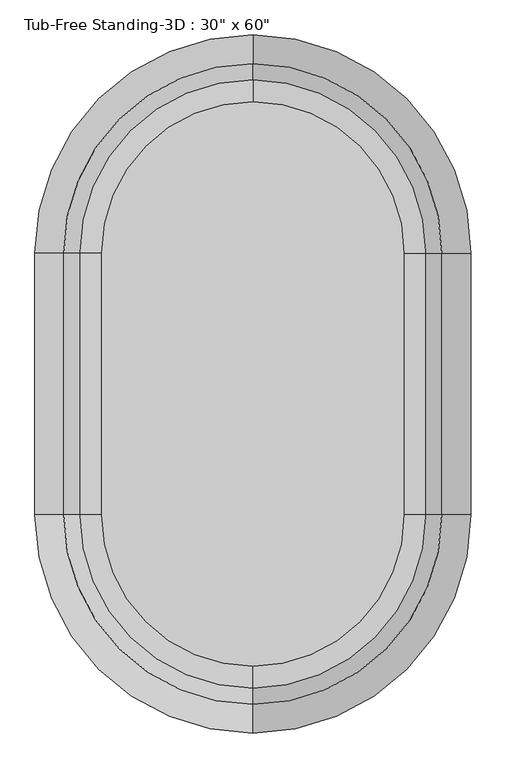
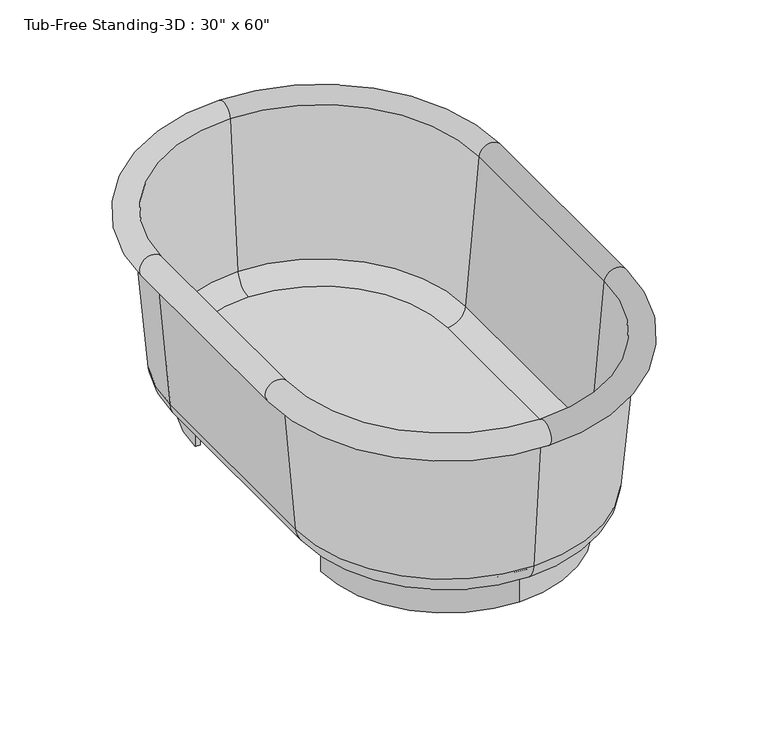
"""IFC4 building model written with IfcOpenShell, lengths in millimetres: flow terminal geometry."""

from ifc_helpers import new_model, si_unit, point, frame, frame_2d, origin, origin_with_axes, place, context, project, spatial, polyline, circle_curve, ellipse_curve, trimmed, segment, composite_curve, outline, extrude, source, transform, mapped, element, save
from ifc_brep_helpers import plane_surface, cylinder_surface, revolved_surface, advanced_brep


def flow_terminal_04541809(model_context):
    return source(origin(), model_context, "Body", "SolidModel", [
        extrude(outline(composite_curve([segment(trimmed(circle_curve(frame_2d((0.0, 228.6)), 254.0), [point((0.0, 482.6))], [point((-254.0, 228.6))], True, "CARTESIAN"), True, "CONTINUOUS"), segment(polyline([(-254.0, 228.6), (-264.2824236, 228.6)]), True, "CONTINUOUS"), segment(trimmed(circle_curve(frame_2d((0.0, 228.6)), 264.2824236), [point((-264.2824236, 228.6))], [point((0.0, 492.8824236))], False, "CARTESIAN"), True, "CONTINUOUS"), segment(trimmed(circle_curve(frame_2d((0.0, 228.6)), 264.2824236), [point((0.0, 492.8824236))], [point((264.2824236, 228.6))], False, "CARTESIAN"), True, "CONTINUOUS"), segment(polyline([(264.2824236, 228.6), (254.0, 228.6)]), True, "CONTINUOUS"), segment(trimmed(circle_curve(frame_2d((0.0, 228.6)), 254.0), [point((254.0, 228.6))], [point((0.0, 482.6))], True, "CARTESIAN"), True, "CONTINUOUS")], self_intersect=False)), origin_with_axes(), (0.0, 0.0, 1.0), 63.5),
        extrude(outline(composite_curve([segment(trimmed(circle_curve(frame_2d((0.0, -228.6)), 264.2824236), [point((0.0, -492.8824236))], [point((-264.2824236, -228.6))], False, "CARTESIAN"), True, "CONTINUOUS"), segment(polyline([(-264.2824236, -228.6), (-254.0, -228.6)]), True, "CONTINUOUS"), segment(trimmed(circle_curve(frame_2d((0.0, -228.6)), 254.0), [point((-254.0, -228.6))], [point((0.0, -482.6))], True, "CARTESIAN"), True, "CONTINUOUS"), segment(trimmed(circle_curve(frame_2d((0.0, -228.6)), 254.0), [point((0.0, -482.6))], [point((254.0, -228.6))], True, "CARTESIAN"), True, "CONTINUOUS"), segment(polyline([(254.0, -228.6), (264.2824236, -228.6)]), True, "CONTINUOUS"), segment(trimmed(circle_curve(frame_2d((0.0, -228.6)), 264.2824236), [point((264.2824236, -228.6))], [point((0.0, -492.8824236))], False, "CARTESIAN"), True, "CONTINUOUS")], self_intersect=False)), origin_with_axes(), (0.0, 0.0, 1.0), 63.5),
        extrude(outline(composite_curve([segment(polyline([(-264.2824236, -228.6), (-264.2824236, 228.6)]), True, "CONTINUOUS"), segment(trimmed(circle_curve(frame_2d((0.0, 228.6)), 264.2824236), [point((-264.2824236, 228.6))], [point((0.0, 492.8824236))], False, "CARTESIAN"), True, "CONTINUOUS"), segment(trimmed(circle_curve(frame_2d((0.0, 228.6)), 264.2824236), [point((0.0, 492.8824236))], [point((264.2824236, 228.6))], False, "CARTESIAN"), True, "CONTINUOUS"), segment(polyline([(264.2824236, 228.6), (264.2824236, -228.6)]), True, "CONTINUOUS"), segment(trimmed(circle_curve(frame_2d((0.0, -228.6)), 264.2824236), [point((264.2824236, -228.6))], [point((0.0, -492.8824236))], False, "CARTESIAN"), True, "CONTINUOUS"), segment(trimmed(circle_curve(frame_2d((0.0, -228.6)), 264.2824236), [point((0.0, -492.8824236))], [point((-264.2824236, -228.6))], False, "CARTESIAN"), True, "CONTINUOUS")], self_intersect=False)), frame((0.0, 0.0, 63.5), z_axis=(0.0, 0.0, 1.0), x_axis=(1.0, 0.0, 0.0)), (0.0, 0.0, 1.0), 15.08125),
        advanced_brep(
        [(0.0, -571.5, 406.4), (342.9, -228.6, 406.4), (355.6, -228.6, 406.4), (0.0, -584.2, 406.4), (0.0, -545.7045038, 111.5561295), (317.1045038, -228.6, 111.5561295), (0.0, -492.8824236, 63.1536107), (264.2824236, -228.6, 63.1536107), (0.0, -492.8824236, 78.0774627), (264.2824236, -228.6, 78.0774627), (0.0, -530.8374416, 112.8568289), (302.2374416, -228.6, 112.8568289), (0.0, -559.0561556, 435.3982063), (330.4561556, -228.6, 435.3982063), (-342.9, -228.6, 406.4), (-355.6, -228.6, 406.4), (-317.1045038, -228.6, 111.5561295), (-264.2824236, -228.6, 63.1536107), (-264.2824236, -228.6, 78.0774627), (-302.2374416, -228.6, 112.8568289), (-330.4561556, -228.6, 435.3982063), (-355.6, 228.6, 406.4), (-342.9, 228.6, 406.4), (-317.1045038, 228.6, 111.5561295), (-264.2824236, 228.6, 63.1536107), (-264.2824236, 228.6, 78.0774627), (-302.2374416, 228.6, 112.8568289), (-330.4561556, 228.6, 435.3982063), (0.0, 571.5, 406.4), (0.0, 584.2, 406.4), (0.0, 545.7045038, 111.5561295), (0.0, 492.8824236, 63.1536107), (0.0, 492.8824236, 78.0774627), (0.0, 530.8374416, 112.8568289), (0.0, 559.0561556, 435.3982063), (342.9, 228.6, 406.4), (355.6, 228.6, 406.4), (317.1045038, 228.6, 111.5561295), (264.2824236, 228.6, 63.1536107), (264.2824236, 228.6, 78.0774627), (302.2374416, 228.6, 112.8568289), (330.4561556, 228.6, 435.3982063)],
        [
            (0, 1, circle_curve(frame((0.0, -228.6, 406.4), z_axis=(0.0, 0.0, 1.0), x_axis=(1.0, 0.0, 0.0)), 342.9)),
            (1, 2),
            (2, 3, circle_curve(frame((0.0, -228.6, 406.4), z_axis=(0.0, 0.0, -1.0), x_axis=(1.0, 0.0, 0.0)), 355.6)),
            (3, 0),
            (4, 5, circle_curve(frame((0.0, -228.6, 111.5561295), z_axis=(0.0, 0.0, 1.0), x_axis=(1.0, 0.0, 0.0)), 317.1045038)),
            (5, 1),
            (0, 4),
            (6, 7, circle_curve(frame((0.0, -228.6, 63.1536107), z_axis=(0.0, 0.0, 1.0), x_axis=(1.0, 0.0, 0.0)), 264.2824236)),
            (7, 5, circle_curve(frame((264.2824236, -228.6, 116.1774627), z_axis=(0.0, -1.0, 0.0), x_axis=(1.0, 0.0, 0.0)), 53.023852)),
            (4, 6, circle_curve(frame((0.0, -492.8824236, 116.1774627), z_axis=(1.0, 0.0, 0.0), x_axis=(0.0, -1.0, 0.0)), 53.023852)),
            (8, 9, circle_curve(frame((0.0, -228.6, 78.0774627), z_axis=(0.0, 0.0, 1.0), x_axis=(1.0, 0.0, 0.0)), 264.2824236)),
            (9, 7),
            (6, 8),
            (10, 11, circle_curve(frame((0.0, -228.6, 112.8568289), z_axis=(0.0, 0.0, 1.0), x_axis=(1.0, 0.0, 0.0)), 302.2374416)),
            (11, 9, circle_curve(frame((264.2824236, -228.6, 116.1774627), z_axis=(0.0, 1.0, 0.0), x_axis=(1.0, 0.0, 0.0)), 38.1)),
            (8, 10, circle_curve(frame((0.0, -492.8824236, 116.1774627), z_axis=(-1.0, 0.0, 0.0), x_axis=(0.0, -1.0, 0.0)), 38.1)),
            (12, 13, circle_curve(frame((0.0, -228.6, 435.3982063), z_axis=(0.0, 0.0, 1.0), x_axis=(1.0, 0.0, 0.0)), 330.4561556)),
            (13, 11),
            (10, 12),
            (2, 13, circle_curve(frame((355.6, -228.6, 431.8), z_axis=(0.0, -1.0, 0.0), x_axis=(1.0, 0.0, 0.0)), 25.4)),
            (12, 3, circle_curve(frame((0.0, -584.2, 431.8), z_axis=(1.0, 0.0, 0.0), x_axis=(0.0, -1.0, 0.0)), 25.4)),
            (14, 0, circle_curve(frame((0.0, -228.6, 406.4), z_axis=(0.0, 0.0, 1.0), x_axis=(0.0, -1.0, 0.0)), 342.9)),
            (3, 15, circle_curve(frame((0.0, -228.6, 406.4), z_axis=(0.0, 0.0, -1.0), x_axis=(0.0, -1.0, 0.0)), 355.6)),
            (15, 14),
            (16, 4, circle_curve(frame((0.0, -228.6, 111.5561295), z_axis=(0.0, 0.0, 1.0), x_axis=(0.0, -1.0, 0.0)), 317.1045038)),
            (14, 16),
            (17, 6, circle_curve(frame((0.0, -228.6, 63.1536107), z_axis=(0.0, 0.0, 1.0), x_axis=(0.0, -1.0, 0.0)), 264.2824236)),
            (16, 17, circle_curve(frame((-264.2824236, -228.6, 116.1774627), z_axis=(0.0, -1.0, 0.0), x_axis=(-1.0, 0.0, 0.0)), 53.023852)),
            (18, 8, circle_curve(frame((0.0, -228.6, 78.0774627), z_axis=(0.0, 0.0, 1.0), x_axis=(0.0, -1.0, 0.0)), 264.2824236)),
            (17, 18),
            (19, 10, circle_curve(frame((0.0, -228.6, 112.8568289), z_axis=(0.0, 0.0, 1.0), x_axis=(0.0, -1.0, 0.0)), 302.2374416)),
            (18, 19, circle_curve(frame((-264.2824236, -228.6, 116.1774627), z_axis=(0.0, 1.0, 0.0), x_axis=(-1.0, 0.0, 0.0)), 38.1)),
            (20, 12, circle_curve(frame((0.0, -228.6, 435.3982063), z_axis=(0.0, 0.0, 1.0), x_axis=(0.0, -1.0, 0.0)), 330.4561556)),
            (19, 20),
            (20, 15, circle_curve(frame((-355.6, -228.6, 431.8), z_axis=(0.0, -1.0, 0.0), x_axis=(-1.0, 0.0, 0.0)), 25.4)),
            (15, 21),
            (21, 22),
            (22, 14),
            (22, 23),
            (23, 16),
            (23, 24, circle_curve(frame((-264.2824236, 228.6, 116.1774627), z_axis=(0.0, -1.0, 0.0), x_axis=(-1.0, 0.0, 0.0)), 53.023852)),
            (24, 17),
            (24, 25),
            (25, 18),
            (25, 26, circle_curve(frame((-264.2824236, 228.6, 116.1774627), z_axis=(0.0, 1.0, 0.0), x_axis=(-1.0, 0.0, 0.0)), 38.1)),
            (26, 19),
            (26, 27),
            (27, 20),
            (27, 21, circle_curve(frame((-355.6, 228.6, 431.8), z_axis=(0.0, -1.0, 0.0), x_axis=(-1.0, 0.0, 0.0)), 25.4)),
            (28, 22, circle_curve(frame((0.0, 228.6, 406.4), z_axis=(0.0, 0.0, 1.0), x_axis=(-1.0, 0.0, 0.0)), 342.9)),
            (21, 29, circle_curve(frame((0.0, 228.6, 406.4), z_axis=(0.0, 0.0, -1.0), x_axis=(-1.0, 0.0, 0.0)), 355.6)),
            (29, 28),
            (30, 23, circle_curve(frame((0.0, 228.6, 111.5561295), z_axis=(0.0, 0.0, 1.0), x_axis=(-1.0, 0.0, 0.0)), 317.1045038)),
            (28, 30),
            (31, 24, circle_curve(frame((0.0, 228.6, 63.1536107), z_axis=(0.0, 0.0, 1.0), x_axis=(-1.0, 0.0, 0.0)), 264.2824236)),
            (30, 31, circle_curve(frame((0.0, 492.8824236, 116.1774627), z_axis=(-1.0, 0.0, 0.0), x_axis=(0.0, 1.0, 0.0)), 53.023852)),
            (32, 25, circle_curve(frame((0.0, 228.6, 78.0774627), z_axis=(0.0, 0.0, 1.0), x_axis=(-1.0, 0.0, 0.0)), 264.2824236)),
            (31, 32),
            (33, 26, circle_curve(frame((0.0, 228.6, 112.8568289), z_axis=(0.0, 0.0, 1.0), x_axis=(-1.0, 0.0, 0.0)), 302.2374416)),
            (32, 33, circle_curve(frame((0.0, 492.8824236, 116.1774627), z_axis=(1.0, 0.0, 0.0), x_axis=(0.0, 1.0, 0.0)), 38.1)),
            (34, 27, circle_curve(frame((0.0, 228.6, 435.3982063), z_axis=(0.0, 0.0, 1.0), x_axis=(-1.0, 0.0, 0.0)), 330.4561556)),
            (33, 34),
            (34, 29, circle_curve(frame((0.0, 584.2, 431.8), z_axis=(-1.0, 0.0, 0.0), x_axis=(0.0, 1.0, 0.0)), 25.4)),
            (35, 28, circle_curve(frame((0.0, 228.6, 406.4), z_axis=(0.0, 0.0, 1.0), x_axis=(0.0, 1.0, 0.0)), 342.9)),
            (29, 36, circle_curve(frame((0.0, 228.6, 406.4), z_axis=(0.0, 0.0, -1.0), x_axis=(0.0, 1.0, 0.0)), 355.6)),
            (36, 35),
            (37, 30, circle_curve(frame((0.0, 228.6, 111.5561295), z_axis=(0.0, 0.0, 1.0), x_axis=(0.0, 1.0, 0.0)), 317.1045038)),
            (35, 37),
            (38, 31, circle_curve(frame((0.0, 228.6, 63.1536107), z_axis=(0.0, 0.0, 1.0), x_axis=(0.0, 1.0, 0.0)), 264.2824236)),
            (37, 38, circle_curve(frame((264.2824236, 228.6, 116.1774627), z_axis=(0.0, 1.0, 0.0), x_axis=(1.0, 0.0, 0.0)), 53.023852)),
            (39, 32, circle_curve(frame((0.0, 228.6, 78.0774627), z_axis=(0.0, 0.0, 1.0), x_axis=(0.0, 1.0, 0.0)), 264.2824236)),
            (38, 39),
            (40, 33, circle_curve(frame((0.0, 228.6, 112.8568289), z_axis=(0.0, 0.0, 1.0), x_axis=(0.0, 1.0, 0.0)), 302.2374416)),
            (39, 40, circle_curve(frame((264.2824236, 228.6, 116.1774627), z_axis=(0.0, -1.0, 0.0), x_axis=(1.0, 0.0, 0.0)), 38.1)),
            (41, 34, circle_curve(frame((0.0, 228.6, 435.3982063), z_axis=(0.0, 0.0, 1.0), x_axis=(0.0, 1.0, 0.0)), 330.4561556)),
            (40, 41),
            (41, 36, circle_curve(frame((355.6, 228.6, 431.8), z_axis=(0.0, 1.0, 0.0), x_axis=(1.0, 0.0, 0.0)), 25.4)),
            (36, 2),
            (1, 35),
            (5, 37),
            (7, 38),
            (9, 39),
            (11, 40),
            (13, 41),
        ],
        [
            plane_surface(frame((0.0, -228.6, 406.4), z_axis=(0.0, 0.0, -1.0), x_axis=(1.0, 0.0, 0.0))),
            revolved_surface(polyline([(342.9, -228.6, 406.4), (317.1045038, -228.6, 111.5561295)]), (0.0, -228.6, 431.8), (0.0, 0.0, -1.0)),
            revolved_surface(trimmed(ellipse_curve(frame((264.2824236, -228.6, 116.1774627), z_axis=(0.0, 1.0, 0.0), x_axis=(1.0, 0.0, 0.0)), 53.023852, 53.023852), [point((317.1045038, -228.6, 111.5561295))], [point((264.2824236, -228.6, 63.1536107))], True, "CARTESIAN"), (0.0, -228.6, 431.8), (0.0, 0.0, -1.0)),
            revolved_surface(polyline([(264.2824236, -228.6, 63.1536107), (264.2824236, -228.6, 78.07746270000001)]), (0.0, -228.6, 431.8), (0.0, 0.0, -1.0)),
            revolved_surface(trimmed(ellipse_curve(frame((264.2824236, -228.6, 116.1774627), z_axis=(0.0, -1.0, 0.0), x_axis=(1.0, 0.0, 0.0)), 38.1, 38.1), [point((264.2824236, -228.6, 78.0774627))], [point((302.2374416, -228.6, 112.8568289))], True, "CARTESIAN"), (0.0, -228.6, 431.8), (0.0, 0.0, -1.0)),
            revolved_surface(polyline([(302.2374416, -228.6, 112.8568289), (330.4561556, -228.6, 435.3982063)]), (0.0, -228.6, 431.8), (0.0, 0.0, -1.0)),
            revolved_surface(trimmed(ellipse_curve(frame((355.6, -228.6, 431.8), z_axis=(0.0, 1.0, 0.0), x_axis=(1.0, 0.0, 0.0)), 25.4, 25.4), [point((330.4561556, -228.6, 435.3982063))], [point((355.6, -228.6, 406.4))], True, "CARTESIAN"), (0.0, -228.6, 431.8), (0.0, 0.0, -1.0)),
            plane_surface(frame((0.0, -228.6, 406.4), z_axis=(0.0, 0.0, -1.0), x_axis=(0.0, -1.0, 0.0))),
            revolved_surface(polyline([(0.0, -571.5, 406.4), (0.0, -545.7045038, 111.5561295)]), (0.0, -228.6, 431.8), (0.0, 0.0, -1.0)),
            revolved_surface(trimmed(ellipse_curve(frame((0.0, -492.8824236, 116.1774627), z_axis=(1.0, 0.0, 0.0), x_axis=(0.0, -1.0, 0.0)), 53.023852, 53.023852), [point((0.0, -545.7045038, 111.5561295))], [point((0.0, -492.8824236, 63.1536107))], True, "CARTESIAN"), (0.0, -228.6, 431.8), (0.0, 0.0, -1.0)),
            revolved_surface(polyline([(0.0, -492.88242360000004, 63.1536107), (0.0, -492.88242360000004, 78.07746270000001)]), (0.0, -228.6, 431.8), (0.0, 0.0, -1.0)),
            revolved_surface(trimmed(ellipse_curve(frame((0.0, -492.8824236, 116.1774627), z_axis=(-1.0, 0.0, 0.0), x_axis=(0.0, -1.0, 0.0)), 38.1, 38.1), [point((0.0, -492.8824236, 78.0774627))], [point((0.0, -530.8374416, 112.8568289))], True, "CARTESIAN"), (0.0, -228.6, 431.8), (0.0, 0.0, -1.0)),
            revolved_surface(polyline([(0.0, -530.8374416, 112.8568289), (0.0, -559.0561556, 435.3982063)]), (0.0, -228.6, 431.8), (0.0, 0.0, -1.0)),
            revolved_surface(trimmed(ellipse_curve(frame((0.0, -584.2, 431.8), z_axis=(1.0, 0.0, 0.0), x_axis=(0.0, -1.0, 0.0)), 25.4, 25.4), [point((0.0, -559.0561556, 435.3982063))], [point((0.0, -584.2, 406.4))], True, "CARTESIAN"), (0.0, -228.6, 431.8), (0.0, 0.0, -1.0)),
            plane_surface(frame((-355.6, -228.6, 406.4), z_axis=(0.0, 0.0, -1.0), x_axis=(0.0, 1.0, 0.0))),
            plane_surface(frame((-342.9, -228.6, 406.4), z_axis=(-0.9961946980917455, 0.0, -0.08715574274765871), x_axis=(0.0, 1.0, 0.0))),
            cylinder_surface(frame((-264.2824236, -228.6, 116.1774627), z_axis=(0.0, -1.0, 0.0), x_axis=(-1.0, 0.0, 0.0)), 53.023852),
            plane_surface(frame((-264.2824236, -228.6, 63.1536107), z_axis=(1.0, 0.0, 0.0), x_axis=(0.0, 1.0, 0.0))),
            revolved_surface(polyline([(-302.38242360000004, 228.6, 116.1774627), (-302.38242360000004, -228.6, 116.1774627)]), (-264.2824236, -228.6, 116.1774627), (0.0, 1.0, 0.0)),
            plane_surface(frame((-302.2374416, -228.6, 112.8568289), z_axis=(0.9961946980917458, 0.0, 0.08715574274765651), x_axis=(0.0, 1.0, 0.0))),
            cylinder_surface(frame((-355.6, -228.6, 431.8), z_axis=(0.0, -1.0, 0.0), x_axis=(-1.0, 0.0, 0.0)), 25.4),
            plane_surface(frame((0.0, 228.6, 406.4), z_axis=(0.0, 0.0, -1.0), x_axis=(-1.0, 0.0, 0.0))),
            revolved_surface(polyline([(-342.9, 228.6, 406.4), (-317.1045038, 228.6, 111.5561295)]), (0.0, 228.6, 431.8), (0.0, 0.0, -1.0)),
            revolved_surface(trimmed(ellipse_curve(frame((-264.2824236, 228.6, 116.1774627), z_axis=(0.0, -1.0, 0.0), x_axis=(-1.0, 0.0, 0.0)), 53.023852, 53.023852), [point((-317.1045038, 228.6, 111.5561295))], [point((-264.2824236, 228.6, 63.1536107))], True, "CARTESIAN"), (0.0, 228.6, 431.8), (0.0, 0.0, -1.0)),
            revolved_surface(polyline([(-264.2824236, 228.6, 63.1536107), (-264.2824236, 228.6, 78.07746270000001)]), (0.0, 228.6, 431.8), (0.0, 0.0, -1.0)),
            revolved_surface(trimmed(ellipse_curve(frame((-264.2824236, 228.6, 116.1774627), z_axis=(0.0, 1.0, 0.0), x_axis=(-1.0, 0.0, 0.0)), 38.1, 38.1), [point((-264.2824236, 228.6, 78.0774627))], [point((-302.2374416, 228.6, 112.8568289))], True, "CARTESIAN"), (0.0, 228.6, 431.8), (0.0, 0.0, -1.0)),
            revolved_surface(polyline([(-302.2374416, 228.6, 112.8568289), (-330.4561556, 228.6, 435.3982063)]), (0.0, 228.6, 431.8), (0.0, 0.0, -1.0)),
            revolved_surface(trimmed(ellipse_curve(frame((-355.6, 228.6, 431.8), z_axis=(0.0, -1.0, 0.0), x_axis=(-1.0, 0.0, 0.0)), 25.4, 25.4), [point((-330.4561556, 228.6, 435.3982063))], [point((-355.6, 228.6, 406.4))], True, "CARTESIAN"), (0.0, 228.6, 431.8), (0.0, 0.0, -1.0)),
            plane_surface(frame((0.0, 228.6, 406.4), z_axis=(0.0, 0.0, -1.0), x_axis=(0.0, 1.0, 0.0))),
            revolved_surface(polyline([(0.0, 571.5, 406.4), (0.0, 545.7045038, 111.5561295)]), (0.0, 228.6, 431.8), (0.0, 0.0, -1.0)),
            revolved_surface(trimmed(ellipse_curve(frame((0.0, 492.8824236, 116.1774627), z_axis=(-1.0, 0.0, 0.0), x_axis=(0.0, 1.0, 0.0)), 53.023852, 53.023852), [point((0.0, 545.7045038, 111.5561295))], [point((0.0, 492.8824236, 63.1536107))], True, "CARTESIAN"), (0.0, 228.6, 431.8), (0.0, 0.0, -1.0)),
            revolved_surface(polyline([(0.0, 492.88242360000004, 63.1536107), (0.0, 492.88242360000004, 78.07746270000001)]), (0.0, 228.6, 431.8), (0.0, 0.0, -1.0)),
            revolved_surface(trimmed(ellipse_curve(frame((0.0, 492.8824236, 116.1774627), z_axis=(1.0, 0.0, 0.0), x_axis=(0.0, 1.0, 0.0)), 38.1, 38.1), [point((0.0, 492.8824236, 78.0774627))], [point((0.0, 530.8374416, 112.8568289))], True, "CARTESIAN"), (0.0, 228.6, 431.8), (0.0, 0.0, -1.0)),
            revolved_surface(polyline([(0.0, 530.8374416, 112.8568289), (0.0, 559.0561556, 435.3982063)]), (0.0, 228.6, 431.8), (0.0, 0.0, -1.0)),
            revolved_surface(trimmed(ellipse_curve(frame((0.0, 584.2, 431.8), z_axis=(-1.0, 0.0, 0.0), x_axis=(0.0, 1.0, 0.0)), 25.4, 25.4), [point((0.0, 559.0561556, 435.3982063))], [point((0.0, 584.2, 406.4))], True, "CARTESIAN"), (0.0, 228.6, 431.8), (0.0, 0.0, -1.0)),
            plane_surface(frame((355.6, 228.6, 406.4), z_axis=(0.0, 0.0, -1.0), x_axis=(0.0, -1.0, 0.0))),
            plane_surface(frame((342.9, 228.6, 406.4), z_axis=(0.9961946980917455, 0.0, -0.08715574274765871), x_axis=(0.0, -1.0, 0.0))),
            cylinder_surface(frame((264.2824236, 228.6, 116.1774627), z_axis=(0.0, 1.0, 0.0), x_axis=(1.0, 0.0, 0.0)), 53.023852),
            plane_surface(frame((264.2824236, 228.6, 63.1536107), z_axis=(-1.0, 0.0, 0.0), x_axis=(0.0, -1.0, 0.0))),
            revolved_surface(polyline([(302.38242360000004, -228.6, 116.1774627), (302.38242360000004, 228.6, 116.1774627)]), (264.2824236, 228.6, 116.1774627), (0.0, -1.0, 0.0)),
            plane_surface(frame((302.2374416, 228.6, 112.8568289), z_axis=(-0.9961946980917458, 0.0, 0.08715574274765651), x_axis=(0.0, -1.0, 0.0))),
            cylinder_surface(frame((355.6, 228.6, 431.8), z_axis=(0.0, 1.0, 0.0), x_axis=(1.0, 0.0, 0.0)), 25.4),
        ],
        [
            (0, [[1, 2, 3, 4]]),
            (1, [[5, 6, -1, 7]]),
            (2, [[8, 9, -5, 10]]),
            (3, [[11, 12, -8, 13]]),
            (4, [[14, 15, -11, 16]]),
            (5, [[17, 18, -14, 19]]),
            (6, [[-3, 20, -17, 21]]),
            (7, [[22, -4, 23, 24]]),
            (8, [[25, -7, -22, 26]]),
            (9, [[27, -10, -25, 28]]),
            (10, [[29, -13, -27, 30]]),
            (11, [[31, -16, -29, 32]]),
            (12, [[33, -19, -31, 34]]),
            (13, [[-23, -21, -33, 35]]),
            (14, [[-24, 36, 37, 38]]),
            (15, [[-26, -38, 39, 40]]),
            (16, [[-28, -40, 41, 42]]),
            (17, [[-30, -42, 43, 44]]),
            (18, [[-32, -44, 45, 46]]),
            (19, [[-34, -46, 47, 48]]),
            (20, [[-35, -48, 49, -36]]),
            (21, [[50, -37, 51, 52]]),
            (22, [[53, -39, -50, 54]]),
            (23, [[55, -41, -53, 56]]),
            (24, [[57, -43, -55, 58]]),
            (25, [[59, -45, -57, 60]]),
            (26, [[61, -47, -59, 62]]),
            (27, [[-51, -49, -61, 63]]),
            (28, [[64, -52, 65, 66]]),
            (29, [[67, -54, -64, 68]]),
            (30, [[69, -56, -67, 70]]),
            (31, [[71, -58, -69, 72]]),
            (32, [[73, -60, -71, 74]]),
            (33, [[75, -62, -73, 76]]),
            (34, [[-65, -63, -75, 77]]),
            (35, [[-66, 78, -2, 79]]),
            (36, [[-68, -79, -6, 80]]),
            (37, [[-70, -80, -9, 81]]),
            (38, [[-72, -81, -12, 82]]),
            (39, [[-74, -82, -15, 83]]),
            (40, [[-76, -83, -18, 84]]),
            (41, [[-77, -84, -20, -78]]),
        ],
    ),
    ])


if __name__ == "__main__":
    model = new_model("IFC4")
    model_context = context("Model", 3, world=origin())
    ifc_project = project(units=[si_unit("LENGTHUNIT", "METRE", prefix="MILLI")], contexts=[model_context])
    site = spatial("IfcSite", under=ifc_project)
    building = spatial("IfcBuilding", under=site)
    placement = place(None, origin())
    flow_terminal_shape = flow_terminal_04541809(model_context)
    element("IfcFlowTerminal", 1, ObjectType="Tub-Free Standing-3D : 30\" x 60\"", at=placement, inside=building, context=model_context, shape_type="MappedRepresentation", body=[
        mapped(flow_terminal_shape, transform((0.0, 0.0, 0.0), x_axis=(1.0, 0.0, 0.0), y_axis=(0.0, 1.0, 0.0), z_axis=(0.0, 0.0, 1.0))),
    ])
    save(model, "model.ifc")

# Revit data of these elements
# Type "Tub-Free Standing-3D : 30\" x 60\""
#   Assembly Code = "D2010110"
#   Height = 1' - 6"
#   Length = 4' - 0"
#   Width = 2' - 6"
#   Tub Material = Porcelain, Ivory
#   Default Elevation = 0
# Element 1 (IfcFlowTerminal, "Tub-Free Standing-3D : 30\" x 60\"")
#   Materials on its faces: "Porcelain, Ivory"
# Materials
#   "Porcelain, Ivory": class "Ceramic", colour RGB 247 247 239, transparency 0, Description = "Porcelain, ivory", Cost = 0
